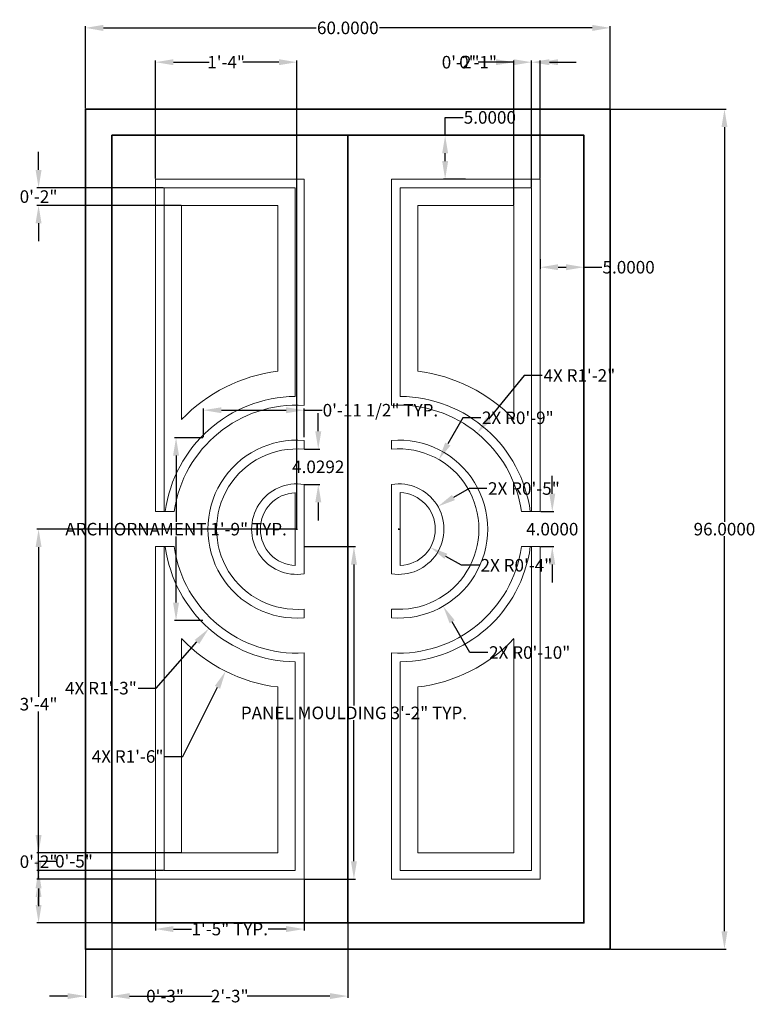
# Model space of a CAD drawing. Units: inches. Extents: x 387 to 471, y 415 to 527.
import ezdxf

# ---------------------------------------------------------------- set-up
doc = ezdxf.new("R2010")
doc.units = ezdxf.units.IN
doc.header["$MEASUREMENT"] = 0
for name, color, linetype, lineweight in [('A-ANNO-DIMS', 2, 'Continuous', 18), ('A-DOOR', 4, 'Continuous', 35), ('A-DOOR-DETL', 3, 'Continuous', 18)]:
    doc.layers.add(name, color=color, linetype=linetype, lineweight=lineweight)
doc.styles.get("Standard").update_dxf_attribs({"font": 'arial.ttf'})
doc.dimstyles.get("Standard").update_dxf_attribs({"dimtxt": 1.433, "dimasz": 2.052, "dimexe": 0.18, "dimexo": 0.0625, "dimgap": 0.09, "dimtad": 0, "dimtih": 1, "dimtoh": 1, "dimdec": 4, "dimzin": 0, "dimdsep": 46, "dimtxsty": 'Standard', "dimcen": 0.09, "dimadec": 0, "dimazin": 0, "dimtfac": 1, "dimtdec": 4, "dimtofl": 0, "dimtmove": 0, "dimatfit": 3, "dimfxl": 1, "dimtolj": 1, "dimtzin": 0, "dimarcsym": 0})

# ---------------------------------------------------------------- blocks, each defined once
blk = doc.blocks.new('*D1')
at = {"layer": 'A-ANNO-DIMS', "color": 0, "lineweight": -2, "transparency": 16777216}
for p, q in [((394.74, 517.13), (394.74, 526.53)), ((396.79, 526.35), (421.12, 526.35)), ((452.69, 526.35), (428.36, 526.35)), ((454.74, 517.13), (454.74, 526.53))]:
    blk.add_line(p, q, dxfattribs=at)
at = {"layer": 'A-ANNO-DIMS', "color": 0, "transparency": 16777216}
for points in [[(396.79, 526.69), (396.79, 526), (394.74, 526.35)], [(452.69, 526.69), (452.69, 526), (454.74, 526.35)]]:
    blk.add_solid(points, dxfattribs=at)
at = {"layer": 'Defpoints', "color": 0, "transparency": 16777216}
for p in [(454.74, 526.35), (394.74, 517.07), (454.74, 517.07)]:
    blk.add_point(p, dxfattribs=at)
at = {"layer": 'A-ANNO-DIMS', "color": 0, "transparency": 16777216, "insert": (424.74, 526.35), "char_height": 1.433, "attachment_point": 5}
blk.add_mtext('\\A1;60.0000', dxfattribs=at)
blk = doc.blocks.new('*D2')
at = {"layer": 'A-ANNO-DIMS', "color": 0, "lineweight": -2, "transparency": 16777216}
for p, q in [((435.87, 514.07), (435.87, 516.12)), ((435.87, 516.12), (437.92, 516.12)), ((438.18, 514.07), (435.69, 514.07)), ((435.87, 511.12), (435.87, 512.02)), ((438.18, 509.07), (435.69, 509.07))]:
    blk.add_line(p, q, dxfattribs=at)
at = {"layer": 'A-ANNO-DIMS', "color": 0, "transparency": 16777216}
for points in [[(435.53, 512.02), (436.21, 512.02), (435.87, 514.07)], [(435.53, 511.12), (436.21, 511.12), (435.87, 509.07)]]:
    blk.add_solid(points, dxfattribs=at)
at = {"layer": 'Defpoints', "color": 0, "transparency": 16777216}
for p in [(435.87, 514.07), (438.24, 514.07), (438.24, 509.07)]:
    blk.add_point(p, dxfattribs=at)
at = {"layer": 'A-ANNO-DIMS', "color": 0, "transparency": 16777216, "insert": (440.98, 516.12), "char_height": 1.433, "attachment_point": 5}
blk.add_mtext('\\A1;5.0000', dxfattribs=at)
blk = doc.blocks.new('*D3')
at = {"layer": 'A-ANNO-DIMS', "color": 0, "lineweight": -2, "transparency": 16777216}
for p, q in [((446.74, 499.93), (446.74, 498.82)), ((451.74, 499.93), (451.74, 498.82)), ((448.79, 499), (449.69, 499)), ((451.74, 499), (453.79, 499))]:
    blk.add_line(p, q, dxfattribs=at)
at = {"layer": 'A-ANNO-DIMS', "color": 0, "transparency": 16777216}
for points in [[(448.79, 499.34), (448.79, 498.66), (446.74, 499)], [(449.69, 499.34), (449.69, 498.66), (451.74, 499)]]:
    blk.add_solid(points, dxfattribs=at)
at = {"layer": 'Defpoints', "color": 0, "transparency": 16777216}
for p in [(446.74, 500), (451.74, 500), (451.74, 499)]:
    blk.add_point(p, dxfattribs=at)
at = {"layer": 'A-ANNO-DIMS', "color": 0, "transparency": 16777216, "insert": (456.85, 499), "char_height": 1.433, "attachment_point": 5}
blk.add_mtext('\\A1;5.0000', dxfattribs=at)
blk = doc.blocks.new('*D4')
at = {"layer": 'A-ANNO-DIMS', "color": 0, "lineweight": -2, "transparency": 16777216}
for p, q in [((448.12, 473.12), (448.12, 475.18)), ((446.8, 471.07), (448.3, 471.07)), ((446.8, 467.07), (448.3, 467.07)), ((448.12, 465.02), (448.12, 462.97))]:
    blk.add_line(p, q, dxfattribs=at)
at = {"layer": 'A-ANNO-DIMS', "color": 0, "transparency": 16777216}
for points in [[(447.78, 473.12), (448.46, 473.12), (448.12, 471.07)], [(447.78, 465.02), (448.46, 465.02), (448.12, 467.07)]]:
    blk.add_solid(points, dxfattribs=at)
at = {"layer": 'Defpoints', "color": 0, "transparency": 16777216}
for p in [(446.74, 471.07), (448.12, 471.07), (446.74, 467.07)]:
    blk.add_point(p, dxfattribs=at)
at = {"layer": 'A-ANNO-DIMS', "color": 0, "transparency": 16777216, "insert": (448.12, 469.07), "char_height": 1.433, "attachment_point": 5}
blk.add_mtext('\\A1;4.0000', dxfattribs=at)
blk = doc.blocks.new('*D5')
at = {"layer": 'A-ANNO-DIMS', "color": 0, "lineweight": -2, "transparency": 16777216}
for p, q in [((454.8, 517.07), (467.99, 517.07)), ((467.81, 515.02), (467.81, 469.89)), ((467.81, 423.12), (467.81, 468.25)), ((454.8, 421.07), (467.99, 421.07))]:
    blk.add_line(p, q, dxfattribs=at)
at = {"layer": 'A-ANNO-DIMS', "color": 0, "transparency": 16777216}
for points in [[(467.47, 515.02), (468.15, 515.02), (467.81, 517.07)], [(467.47, 423.12), (468.15, 423.12), (467.81, 421.07)]]:
    blk.add_solid(points, dxfattribs=at)
at = {"layer": 'Defpoints', "color": 0, "transparency": 16777216}
for p in [(454.74, 517.07), (454.74, 421.07), (467.81, 421.07)]:
    blk.add_point(p, dxfattribs=at)
at = {"layer": 'A-ANNO-DIMS', "color": 0, "transparency": 16777216, "insert": (467.81, 469.07), "char_height": 1.433, "attachment_point": 5}
blk.add_mtext('\\A1;96.0000', dxfattribs=at)
blk = doc.blocks.new('*D6')
at = {"layer": 'A-ANNO-DIMS', "color": 0, "lineweight": -2, "transparency": 16777216}
for p, q in [((421.36, 480.26), (421.36, 482.31)), ((419.8, 478.21), (421.54, 478.21)), ((419.8, 474.18), (421.54, 474.18)), ((421.36, 472.13), (421.36, 470.07))]:
    blk.add_line(p, q, dxfattribs=at)
at = {"layer": 'A-ANNO-DIMS', "color": 0, "transparency": 16777216}
for points in [[(421.02, 480.26), (421.71, 480.26), (421.36, 478.21)], [(421.02, 472.13), (421.71, 472.13), (421.36, 474.18)]]:
    blk.add_solid(points, dxfattribs=at)
at = {"layer": 'Defpoints', "color": 0, "transparency": 16777216}
for p in [(419.74, 478.21), (419.74, 474.18), (421.36, 474.18)]:
    blk.add_point(p, dxfattribs=at)
at = {"layer": 'A-ANNO-DIMS', "color": 0, "transparency": 16777216, "insert": (421.36, 476.19), "char_height": 1.433, "attachment_point": 5}
blk.add_mtext('\\A1;4.0292', dxfattribs=at)
blk = doc.blocks.new('DOOR-PANEL-MOULDING')
for p, q in [((0, 38), (2.14, 38)), ((3, 3), (3, 27.48)), ((16, 24.83), (16, 1)), ((17, 25.85), (17, 0)), ((14, 21.96), (14, 3))]:
    blk.add_line(p, q)
for points in [[(17, 0), (0, 0), (0, 38)], [(16, 1), (1, 1), (1, 38)], [(14, 3), (3, 3)]]:
    blk.add_lwpolyline(points)
for radius, start, end in [(15.17, 187.5743, 269.3464), (14.17, 188.1122, 273.3447), (18.17, 223.5421, 263.1323)]:
    blk.add_arc((16.17, 40), radius, start, end)
blk = doc.blocks.new('DOOR-ARCH-ORNAMENT')
for p, q in [((11, 20.31), (11, 19.31)), ((11, 15.28), (11, 5.07)), ((10, 14.34), (10, 6)), ((11, 1.04), (11, 0.03))]:
    blk.add_line(p, q)
for radius, start, end in [(10.17, 85.3376, 274.6624), (9.17, 84.828, 275.172), (5.17, 80.8019, 279.1981), (4.17, 92.3772, 267.6228)]:
    blk.add_arc((10.17, 10.17), radius, start, end)
blk = doc.blocks.new('*D9')
at = {"layer": 'A-ANNO-DIMS', "color": 0, "lineweight": -2, "transparency": 16777216}
for p, q in [((419.8, 467.07), (425.62, 467.07)), ((425.44, 465.02), (425.44, 448.9)), ((425.44, 431.12), (425.44, 447.24)), ((419.8, 429.07), (425.62, 429.07))]:
    blk.add_line(p, q, dxfattribs=at)
at = {"layer": 'A-ANNO-DIMS', "color": 0, "transparency": 16777216}
for points in [[(425.1, 465.02), (425.78, 465.02), (425.44, 467.07)], [(425.1, 431.12), (425.78, 431.12), (425.44, 429.07)]]:
    blk.add_solid(points, dxfattribs=at)
at = {"layer": 'Defpoints', "color": 0, "transparency": 16777216}
for p in [(419.74, 467.07), (425.44, 467.07), (419.74, 429.07)]:
    blk.add_point(p, dxfattribs=at)
at = {"layer": 'A-ANNO-DIMS', "color": 0, "transparency": 16777216, "insert": (425.44, 448.07), "char_height": 1.433, "attachment_point": 5}
blk.add_mtext('\\A1;PANEL MOULDING 3\'-2" TYP.', dxfattribs=at)
blk = doc.blocks.new('*D10')
at = {"layer": 'A-ANNO-DIMS', "color": 0, "lineweight": -2, "transparency": 16777216}
for p, q in [((402.74, 429.01), (402.74, 423.19)), ((419.74, 429.01), (419.74, 423.19)), ((404.79, 423.37), (406.85, 423.37)), ((417.69, 423.37), (415.63, 423.37))]:
    blk.add_line(p, q, dxfattribs=at)
at = {"layer": 'A-ANNO-DIMS', "color": 0, "transparency": 16777216}
for points in [[(404.79, 423.71), (404.79, 423.03), (402.74, 423.37)], [(417.69, 423.71), (417.69, 423.03), (419.74, 423.37)]]:
    blk.add_solid(points, dxfattribs=at)
at = {"layer": 'Defpoints', "color": 0, "transparency": 16777216}
for p in [(402.74, 429.07), (419.74, 429.07), (419.74, 423.37)]:
    blk.add_point(p, dxfattribs=at)
at = {"layer": 'A-ANNO-DIMS', "color": 0, "transparency": 16777216, "insert": (411.24, 423.37), "char_height": 1.433, "attachment_point": 5}
blk.add_mtext('\\A1;1\'-5" TYP.', dxfattribs=at)
blk = doc.blocks.new('*D11')
at = {"layer": 'A-ANNO-DIMS', "color": 0, "lineweight": -2, "transparency": 16777216}
for p, q in [((408.17, 479.52), (404.92, 479.52)), ((405.1, 477.47), (405.1, 469.9)), ((405.1, 460.67), (405.1, 468.24)), ((408.17, 458.62), (404.92, 458.62))]:
    blk.add_line(p, q, dxfattribs=at)
at = {"layer": 'A-ANNO-DIMS', "color": 0, "transparency": 16777216}
for points in [[(404.76, 477.47), (405.44, 477.47), (405.1, 479.52)], [(404.76, 460.67), (405.44, 460.67), (405.1, 458.62)]]:
    blk.add_solid(points, dxfattribs=at)
at = {"layer": 'Defpoints', "color": 0, "transparency": 16777216}
for p in [(405.1, 479.52), (408.24, 479.52), (408.24, 458.62)]:
    blk.add_point(p, dxfattribs=at)
at = {"layer": 'A-ANNO-DIMS', "color": 0, "transparency": 16777216, "insert": (405.1, 469.07), "char_height": 1.433, "attachment_point": 5}
blk.add_mtext('\\A1;ARCH ORNAMENT 1\'-9" TYP.', dxfattribs=at)
blk = doc.blocks.new('*D12')
at = {"layer": 'A-ANNO-DIMS', "color": 0, "lineweight": -2, "transparency": 16777216}
for p, q in [((408.24, 479.59), (408.24, 482.84)), ((419.74, 479.59), (419.74, 482.84)), ((410.29, 482.66), (417.69, 482.66)), ((419.74, 482.66), (421.79, 482.66))]:
    blk.add_line(p, q, dxfattribs=at)
at = {"layer": 'A-ANNO-DIMS', "color": 0, "transparency": 16777216}
for points in [[(410.29, 483), (410.29, 482.32), (408.24, 482.66)], [(417.69, 483), (417.69, 482.32), (419.74, 482.66)]]:
    blk.add_solid(points, dxfattribs=at)
at = {"layer": 'Defpoints', "color": 0, "transparency": 16777216}
for p in [(419.74, 482.66), (408.24, 479.52), (419.74, 479.52)]:
    blk.add_point(p, dxfattribs=at)
at = {"layer": 'A-ANNO-DIMS', "color": 0, "transparency": 16777216, "insert": (428.47, 482.66), "char_height": 1.433, "attachment_point": 5}
blk.add_mtext('\\A1;0\'-11 1/2" TYP.', dxfattribs=at)
blk = doc.blocks.new('*D13')
at = {"layer": 'A-ANNO-DIMS', "color": 0, "lineweight": -2, "transparency": 16777216}
for p, q in [((397.74, 424.01), (397.74, 415.53)), ((394.74, 421.01), (394.74, 415.53)), ((392.69, 415.71), (390.63, 415.71)), ((399.79, 415.71), (401.84, 415.71))]:
    blk.add_line(p, q, dxfattribs=at)
at = {"layer": 'A-ANNO-DIMS', "color": 0, "transparency": 16777216}
for points in [[(392.69, 416.05), (392.69, 415.37), (394.74, 415.71)], [(399.79, 416.05), (399.79, 415.37), (397.74, 415.71)]]:
    blk.add_solid(points, dxfattribs=at)
at = {"layer": 'Defpoints', "color": 0, "transparency": 16777216}
for p in [(397.74, 424.07), (394.74, 421.07), (397.74, 415.71)]:
    blk.add_point(p, dxfattribs=at)
at = {"layer": 'A-ANNO-DIMS', "color": 0, "transparency": 16777216, "insert": (403.84, 415.71), "char_height": 1.433, "attachment_point": 5}
blk.add_mtext('\\A1;0\'-3"', dxfattribs=at)
blk = doc.blocks.new('*D14')
at = {"layer": 'A-ANNO-DIMS', "color": 0, "lineweight": -2, "transparency": 16777216}
for p, q in [((397.74, 424.01), (397.74, 415.53)), ((424.74, 424.01), (424.74, 415.53)), ((399.79, 415.71), (409.23, 415.71)), ((422.69, 415.71), (413.25, 415.71))]:
    blk.add_line(p, q, dxfattribs=at)
at = {"layer": 'A-ANNO-DIMS', "color": 0, "transparency": 16777216}
for points in [[(399.79, 416.05), (399.79, 415.37), (397.74, 415.71)], [(422.69, 416.05), (422.69, 415.37), (424.74, 415.71)]]:
    blk.add_solid(points, dxfattribs=at)
at = {"layer": 'Defpoints', "color": 0, "transparency": 16777216}
for p in [(397.74, 424.07), (424.74, 424.07), (424.74, 415.71)]:
    blk.add_point(p, dxfattribs=at)
at = {"layer": 'A-ANNO-DIMS', "color": 0, "transparency": 16777216, "insert": (411.24, 415.71), "char_height": 1.433, "attachment_point": 5}
blk.add_mtext('\\A1;2\'-3"', dxfattribs=at)
blk = doc.blocks.new('*D15')
at = {"layer": 'A-ANNO-DIMS', "color": 0, "lineweight": -2, "transparency": 16777216}
for p, q in [((389.38, 429.07), (389.38, 431.12)), ((389.38, 431.12), (391.43, 431.12)), ((402.68, 429.07), (389.2, 429.07)), ((389.38, 426.12), (389.38, 427.02)), ((397.68, 424.07), (389.2, 424.07))]:
    blk.add_line(p, q, dxfattribs=at)
at = {"layer": 'A-ANNO-DIMS', "color": 0, "transparency": 16777216}
for points in [[(389.04, 427.02), (389.72, 427.02), (389.38, 429.07)], [(389.04, 426.12), (389.72, 426.12), (389.38, 424.07)]]:
    blk.add_solid(points, dxfattribs=at)
at = {"layer": 'Defpoints', "color": 0, "transparency": 16777216}
for p in [(389.38, 429.07), (402.74, 429.07), (397.74, 424.07)]:
    blk.add_point(p, dxfattribs=at)
at = {"layer": 'A-ANNO-DIMS', "color": 0, "transparency": 16777216, "insert": (393.43, 431.12), "char_height": 1.433, "attachment_point": 5}
blk.add_mtext('\\A1;0\'-5"', dxfattribs=at)
blk = doc.blocks.new('*D16')
at = {"layer": 'A-ANNO-DIMS', "color": 0, "lineweight": -2, "transparency": 16777216}
for p, q in [((443.69, 522.43), (441.63, 522.43)), ((445.74, 508.13), (445.74, 522.61)), ((446.74, 509.13), (446.74, 522.61)), ((448.79, 522.43), (450.84, 522.43))]:
    blk.add_line(p, q, dxfattribs=at)
at = {"layer": 'A-ANNO-DIMS', "color": 0, "transparency": 16777216}
for points in [[(443.69, 522.77), (443.69, 522.09), (445.74, 522.43)], [(448.79, 522.77), (448.79, 522.09), (446.74, 522.43)]]:
    blk.add_solid(points, dxfattribs=at)
at = {"layer": 'Defpoints', "color": 0, "transparency": 16777216}
for p in [(445.74, 522.43), (446.74, 509.07), (445.74, 508.07)]:
    blk.add_point(p, dxfattribs=at)
at = {"layer": 'A-ANNO-DIMS', "color": 0, "transparency": 16777216, "insert": (439.64, 522.43), "char_height": 1.433, "attachment_point": 5}
blk.add_mtext('\\A1;0\'-1"', dxfattribs=at)
blk = doc.blocks.new('*D17')
at = {"layer": 'A-ANNO-DIMS', "color": 0, "lineweight": -2, "transparency": 16777216}
for p, q in [((441.69, 522.43), (439.63, 522.43)), ((443.74, 506.13), (443.74, 522.61)), ((445.74, 508.13), (445.74, 522.61)), ((447.79, 522.43), (449.84, 522.43))]:
    blk.add_line(p, q, dxfattribs=at)
at = {"layer": 'A-ANNO-DIMS', "color": 0, "transparency": 16777216}
for points in [[(441.69, 522.77), (441.69, 522.09), (443.74, 522.43)], [(447.79, 522.77), (447.79, 522.09), (445.74, 522.43)]]:
    blk.add_solid(points, dxfattribs=at)
at = {"layer": 'Defpoints', "color": 0, "transparency": 16777216}
for p in [(443.74, 522.43), (445.74, 508.07), (443.74, 506.07)]:
    blk.add_point(p, dxfattribs=at)
at = {"layer": 'A-ANNO-DIMS', "color": 0, "transparency": 16777216, "insert": (437.64, 522.43), "char_height": 1.433, "attachment_point": 5}
blk.add_mtext('\\A1;0\'-2"', dxfattribs=at)
blk = doc.blocks.new('*D18')
at = {"layer": 'A-ANNO-DIMS', "color": 0, "lineweight": -2, "transparency": 16777216}
for p, q in [((389.378732, 434.123719), (389.378732, 436.175719)), ((405.676232, 432.071719), (389.198732, 432.071719)), ((403.676232, 430.071719), (389.198732, 430.071719)), ((389.378732, 428.019719), (389.378732, 425.967719))]:
    blk.add_line(p, q, dxfattribs=at)
at = {"layer": 'A-ANNO-DIMS', "color": 0, "transparency": 16777216}
for points in [[(389.036732, 434.123719), (389.720732, 434.123719), (389.378732, 432.071719)], [(389.036732, 428.019719), (389.720732, 428.019719), (389.378732, 430.071719)]]:
    blk.add_solid(points, dxfattribs=at)
at = {"layer": 'Defpoints', "color": 0, "transparency": 16777216}
for p in [(389.378732, 432.071719), (405.738732, 432.071719), (403.738732, 430.071719)]:
    blk.add_point(p, dxfattribs=at)
at = {"layer": 'A-ANNO-DIMS', "color": 0, "transparency": 16777216, "insert": (389.378732, 431.071719), "char_height": 1.433, "attachment_point": 5}
blk.add_mtext('\\A1;0\'-2"', dxfattribs=at)
blk = doc.blocks.new('*D19')
at = {"layer": 'A-ANNO-DIMS', "color": 0, "lineweight": -2, "transparency": 16777216}
for p, q in [((389.378732, 510.123719), (389.378732, 512.175719)), ((403.676232, 508.071719), (389.198732, 508.071719)), ((405.676232, 506.071719), (389.198732, 506.071719)), ((389.378732, 504.019719), (389.378732, 501.967719))]:
    blk.add_line(p, q, dxfattribs=at)
at = {"layer": 'A-ANNO-DIMS', "color": 0, "transparency": 16777216}
for points in [[(389.036732, 510.123719), (389.720732, 510.123719), (389.378732, 508.071719)], [(389.036732, 504.019719), (389.720732, 504.019719), (389.378732, 506.071719)]]:
    blk.add_solid(points, dxfattribs=at)
at = {"layer": 'Defpoints', "color": 0, "transparency": 16777216}
for p in [(403.738732, 508.071719), (389.378732, 506.071719), (405.738732, 506.071719)]:
    blk.add_point(p, dxfattribs=at)
at = {"layer": 'A-ANNO-DIMS', "color": 0, "transparency": 16777216, "insert": (389.378732, 507.071719), "char_height": 1.433, "attachment_point": 5}
blk.add_mtext('\\A1;0\'-2"', dxfattribs=at)
blk = doc.blocks.new('*D20')
at = {"layer": 'A-ANNO-DIMS', "color": 0, "lineweight": -2, "transparency": 16777216}
for p, q in [((402.74, 509.13), (402.74, 522.61)), ((404.79, 522.43), (408.9, 522.43)), ((416.86, 522.43), (412.75, 522.43)), ((418.91, 469.13), (418.91, 522.61))]:
    blk.add_line(p, q, dxfattribs=at)
at = {"layer": 'A-ANNO-DIMS', "color": 0, "transparency": 16777216}
for points in [[(404.79, 522.77), (404.79, 522.09), (402.74, 522.43)], [(416.86, 522.77), (416.86, 522.09), (418.91, 522.43)]]:
    blk.add_solid(points, dxfattribs=at)
at = {"layer": 'Defpoints', "color": 0, "transparency": 16777216}
for p in [(402.74, 522.43), (402.74, 509.07), (418.91, 469.07)]:
    blk.add_point(p, dxfattribs=at)
at = {"layer": 'A-ANNO-DIMS', "color": 0, "transparency": 16777216, "insert": (410.83, 522.43), "char_height": 1.433, "attachment_point": 5}
blk.add_mtext('\\A1;1\'-4"', dxfattribs=at)
blk = doc.blocks.new('*D21')
at = {"layer": 'A-ANNO-DIMS', "color": 0, "lineweight": -2, "transparency": 16777216}
for p, q in [((418.85, 469.07), (389.2, 469.07)), ((389.38, 467.02), (389.38, 449.89)), ((389.38, 431.12), (389.38, 448.25)), ((402.68, 429.07), (389.2, 429.07))]:
    blk.add_line(p, q, dxfattribs=at)
at = {"layer": 'A-ANNO-DIMS', "color": 0, "transparency": 16777216}
for points in [[(389.04, 467.02), (389.72, 467.02), (389.38, 469.07)], [(389.04, 431.12), (389.72, 431.12), (389.38, 429.07)]]:
    blk.add_solid(points, dxfattribs=at)
at = {"layer": 'Defpoints', "color": 0, "transparency": 16777216}
for p in [(418.91, 469.07), (389.38, 429.07), (402.74, 429.07)]:
    blk.add_point(p, dxfattribs=at)
at = {"layer": 'A-ANNO-DIMS', "color": 0, "transparency": 16777216, "insert": (389.38, 449.07), "char_height": 1.433, "attachment_point": 5}
blk.add_mtext('\\A1;3\'-4"', dxfattribs=at)
blk = doc.blocks.new('*D22')
at = {"layer": 'A-ANNO-DIMS', "color": 0, "lineweight": -2, "transparency": 16777216}
for p, q in [((418.82, 469.07), (419, 469.07)), ((418.91, 468.98), (418.91, 469.16)), ((405.86, 443.09), (409.84, 451)), ((403.81, 443.09), (405.86, 443.09))]:
    blk.add_line(p, q, dxfattribs=at)
at = {"layer": 'A-ANNO-DIMS', "color": 0, "transparency": 16777216}
blk.add_solid([(409.53, 451.15), (410.14, 450.84), (410.76, 452.83)], dxfattribs=at)
at = {"layer": 'Defpoints', "color": 0, "transparency": 16777216}
for p in [(418.91, 469.07), (410.76, 452.83)]:
    blk.add_point(p, dxfattribs=at)
at = {"layer": 'A-ANNO-DIMS', "color": 0, "transparency": 16777216, "insert": (399.56, 443.09), "char_height": 1.433, "attachment_point": 5}
blk.add_mtext('\\A1;4X R1\'-6"', dxfattribs=at)
blk = doc.blocks.new('*D23')
at = {"layer": 'A-ANNO-DIMS', "color": 0, "lineweight": -2, "transparency": 16777216}
for p, q in [((418.82, 469.07), (419, 469.07)), ((418.91, 468.98), (418.91, 469.16)), ((402.81, 450.9), (407.49, 456.18)), ((400.76, 450.9), (402.81, 450.9))]:
    blk.add_line(p, q, dxfattribs=at)
at = {"layer": 'A-ANNO-DIMS', "color": 0, "transparency": 16777216}
blk.add_solid([(407.23, 456.41), (407.75, 455.95), (408.85, 457.71)], dxfattribs=at)
at = {"layer": 'Defpoints', "color": 0, "transparency": 16777216}
for p in [(418.91, 469.07), (408.85, 457.71)]:
    blk.add_point(p, dxfattribs=at)
at = {"layer": 'A-ANNO-DIMS', "color": 0, "transparency": 16777216, "insert": (396.51, 450.9), "char_height": 1.433, "attachment_point": 5}
blk.add_mtext('\\A1;4X R1\'-3"', dxfattribs=at)
blk = doc.blocks.new('*D24')
at = {"layer": 'A-ANNO-DIMS', "color": 0, "lineweight": -2, "transparency": 16777216}
for p, q in [((444.92, 486.63), (440.84, 481.63)), ((446.97, 486.63), (444.92, 486.63)), ((430.48, 469.07), (430.66, 469.07)), ((430.57, 468.98), (430.57, 469.16))]:
    blk.add_line(p, q, dxfattribs=at)
at = {"layer": 'A-ANNO-DIMS', "color": 0, "transparency": 16777216}
blk.add_solid([(440.57, 481.85), (441.1, 481.42), (439.54, 480.04)], dxfattribs=at)
at = {"layer": 'Defpoints', "color": 0, "transparency": 16777216}
for p in [(439.54, 480.04), (430.57, 469.07)]:
    blk.add_point(p, dxfattribs=at)
at = {"layer": 'A-ANNO-DIMS', "color": 0, "transparency": 16777216, "insert": (451.22, 486.63), "char_height": 1.433, "attachment_point": 5}
blk.add_mtext('\\A1;4X R1\'-2"', dxfattribs=at)
blk = doc.blocks.new('*D25')
at = {"layer": 'A-ANNO-DIMS', "color": 0, "lineweight": -2, "transparency": 16777216}
for p, q in [((430.48, 469.07), (430.66, 469.07)), ((430.57, 468.98), (430.57, 469.16)), ((438.7, 454.97), (436.68, 458.48)), ((440.75, 454.97), (438.7, 454.97))]:
    blk.add_line(p, q, dxfattribs=at)
at = {"layer": 'A-ANNO-DIMS', "color": 0, "transparency": 16777216}
blk.add_solid([(436.97, 458.65), (436.38, 458.31), (435.65, 460.26)], dxfattribs=at)
at = {"layer": 'Defpoints', "color": 0, "transparency": 16777216}
for p in [(430.57, 469.07), (435.65, 460.26)]:
    blk.add_point(p, dxfattribs=at)
at = {"layer": 'A-ANNO-DIMS', "color": 0, "transparency": 16777216, "insert": (445.54, 454.97), "char_height": 1.433, "attachment_point": 5}
blk.add_mtext('\\A1;2X R0\'-10"', dxfattribs=at)
blk = doc.blocks.new('*D26')
at = {"layer": 'A-ANNO-DIMS', "color": 0, "lineweight": -2, "transparency": 16777216}
for p, q in [((437.9, 481.79), (436.17, 478.8)), ((439.95, 481.79), (437.9, 481.79)), ((430.48, 469.07), (430.66, 469.07)), ((430.57, 468.98), (430.57, 469.16))]:
    blk.add_line(p, q, dxfattribs=at)
at = {"layer": 'A-ANNO-DIMS', "color": 0, "transparency": 16777216}
blk.add_solid([(435.88, 478.97), (436.47, 478.62), (435.15, 477.02)], dxfattribs=at)
at = {"layer": 'Defpoints', "color": 0, "transparency": 16777216}
for p in [(435.15, 477.02), (430.57, 469.07)]:
    blk.add_point(p, dxfattribs=at)
at = {"layer": 'A-ANNO-DIMS', "color": 0, "transparency": 16777216, "insert": (444.18, 481.79), "char_height": 1.433, "attachment_point": 5}
blk.add_mtext('\\A1;2X R0\'-9"', dxfattribs=at)
blk = doc.blocks.new('*D27')
at = {"layer": 'A-ANNO-DIMS', "color": 0, "lineweight": -2, "transparency": 16777216}
for p, q in [((438.6, 473.71), (436.82, 472.68)), ((440.65, 473.71), (438.6, 473.71)), ((430.48, 469.07), (430.66, 469.07)), ((430.57, 468.98), (430.57, 469.16))]:
    blk.add_line(p, q, dxfattribs=at)
at = {"layer": 'A-ANNO-DIMS', "color": 0, "transparency": 16777216}
blk.add_solid([(436.65, 472.98), (436.99, 472.39), (435.05, 471.66)], dxfattribs=at)
at = {"layer": 'Defpoints', "color": 0, "transparency": 16777216}
for p in [(435.05, 471.66), (430.57, 469.07)]:
    blk.add_point(p, dxfattribs=at)
at = {"layer": 'A-ANNO-DIMS', "color": 0, "transparency": 16777216, "insert": (444.88, 473.71), "char_height": 1.433, "attachment_point": 5}
blk.add_mtext('\\A1;2X R0\'-5"', dxfattribs=at)
blk = doc.blocks.new('*D28')
at = {"layer": 'A-ANNO-DIMS', "color": 0, "lineweight": -2, "transparency": 16777216}
for p, q in [((430.48, 469.07), (430.66, 469.07)), ((430.57, 468.98), (430.57, 469.16)), ((437.74, 464.94), (435.96, 465.96)), ((439.79, 464.94), (437.74, 464.94))]:
    blk.add_line(p, q, dxfattribs=at)
at = {"layer": 'A-ANNO-DIMS', "color": 0, "transparency": 16777216}
blk.add_solid([(436.13, 466.26), (435.79, 465.67), (434.18, 466.99)], dxfattribs=at)
at = {"layer": 'Defpoints', "color": 0, "transparency": 16777216}
for p in [(430.57, 469.07), (434.18, 466.99)]:
    blk.add_point(p, dxfattribs=at)
at = {"layer": 'A-ANNO-DIMS', "color": 0, "transparency": 16777216, "insert": (444.02, 464.94), "char_height": 1.433, "attachment_point": 5}
blk.add_mtext('\\A1;2X R0\'-4"', dxfattribs=at)

msp = doc.modelspace()

# ---------------------------------------------------------------- linework, layer by layer
at = {"layer": 'A-DOOR'}
msp.add_line((424.73873, 514.07172), (424.73873, 424.07172), dxfattribs=at)
for points in [[(394.73873, 517.07172), (454.73873, 517.07172), (454.73873, 421.07172), (394.73873, 421.07172)], [(397.73873, 514.07172), (451.73873, 514.07172), (451.73873, 424.07172), (397.73873, 424.07172)]]:
    msp.add_lwpolyline(points, close=True, dxfattribs=at)

# ---------------------------------------------------------------- block references
at = {"layer": 'A-DOOR-DETL', "extrusion": (0, 0, -1), "zscale": -1, "rotation": 180}
msp.add_blockref('DOOR-PANEL-MOULDING', (-402.739, 509.07144), dxfattribs=at)
at = {"layer": 'A-DOOR-DETL', "rotation": 180}
for name, p in [('DOOR-PANEL-MOULDING', (446.73846, 509.07144)), ('DOOR-ARCH-ORNAMENT', (440.73846, 479.24444))]:
    msp.add_blockref(name, p, dxfattribs=at)
at = {"layer": 'A-DOOR-DETL'}
for name, p in [('DOOR-ARCH-ORNAMENT', (408.739, 458.899)), ('DOOR-PANEL-MOULDING', (402.739, 429.072))]:
    msp.add_blockref(name, p, dxfattribs=at)
at = {"layer": 'A-DOOR-DETL', "extrusion": (0, 0, -1), "zscale": -1}
msp.add_blockref('DOOR-PANEL-MOULDING', (-446.73846, 429.072), dxfattribs=at)

# ---------------------------------------------------------------- dimensions: what is measured, and where the dimension line sits
at = {"layer": 'A-ANNO-DIMS'}
for base, p1, p2, override, picture, middle in [((454.73873, 526.34552), (394.73873, 517.07172), (454.73873, 517.07172), {"dimclrd": 0, "dimclre": 0, "dimclrt": 0}, '*D1', (424.73873, 526.34552)), ((402.73873, 522.43172), (418.91182, 469.07172), (402.73873, 509.07172), {"dimdec": 1, "dimlfac": 1, "dimrnd": 0, "dimzin": 1, "dimdsep": 46, "dimlunit": 4, "dimfrac": 2}, '*D20', (410.82528, 522.43172)), ((443.73873, 522.43172), (445.73873, 508.07172), (443.73873, 506.07172), {"dimdec": 1, "dimlfac": 1, "dimrnd": 0, "dimzin": 1, "dimdsep": 46, "dimlunit": 4, "dimfrac": 2}, '*D17', (437.64009, 522.43172)), ((445.73873, 522.43172), (446.73873, 509.07172), (445.73873, 508.07172), {"dimdec": 1, "dimlfac": 1, "dimrnd": 0, "dimzin": 1, "dimdsep": 46, "dimlunit": 4, "dimfrac": 2}, '*D16', (439.64009, 522.43172)), ((451.73873, 499.00173), (446.73873, 499.99566), (451.73873, 499.99566), {"dimclrd": 0, "dimclre": 0, "dimclrt": 0}, '*D3', (456.85279, 499.00173)), ((397.73873, 415.71172), (394.73873, 421.07172), (397.73873, 424.07172), {"dimdec": 1, "dimlfac": 1, "dimrnd": 0, "dimzin": 1, "dimdsep": 46, "dimlunit": 4, "dimfrac": 2}, '*D13', (403.83737, 415.71172)), ((424.73873, 415.71172), (397.73873, 424.07172), (424.73873, 424.07172), {"dimdec": 1, "dimlfac": 1, "dimrnd": 0, "dimzin": 1, "dimdsep": 46, "dimlunit": 4, "dimfrac": 2}, '*D14', (411.23873, 415.71172))]:
    dim = msp.add_linear_dim(base=base, p1=p1, p2=p2, dimstyle='Standard', override=override, dxfattribs=at)
    dim.commit()
    dim.dimension.update_dxf_attribs({"geometry": picture, "text_midpoint": middle})
for base, p1, p2, override, picture, middle in [((435.86883, 514.07172), (438.23873, 509.07172), (438.23873, 514.07172), {"dimclrd": 0, "dimclre": 0, "dimclrt": 0}, '*D2', (440.98289, 516.12372)), ((467.81119, 421.07172), (454.73873, 517.07172), (454.73873, 421.07172), {"dimclrd": 0, "dimclre": 0, "dimclrt": 0}, '*D5', (467.81119, 469.07172)), ((389.37873, 506.07172), (403.73873, 508.07172), (405.73873, 506.07172), {"dimdec": 1, "dimlfac": 1, "dimrnd": 0, "dimzin": 1, "dimdsep": 46, "dimlunit": 4, "dimfrac": 2}, '*D19', (389.37873, 507.07172)), ((421.36448, 474.17829), (419.73873, 478.20746), (419.73873, 474.17829), {"dimclrd": 0, "dimclre": 0, "dimclrt": 0}, '*D6', (421.36448, 476.19288)), ((448.12223, 471.07172), (446.73873, 467.07172), (446.73873, 471.07172), {"dimclrd": 0, "dimclre": 0, "dimclrt": 0}, '*D4', (448.12223, 469.07172)), ((389.37873, 429.07172), (418.91182, 469.07172), (402.73873, 429.07172), {"dimdec": 1, "dimlfac": 1, "dimrnd": 0, "dimzin": 1, "dimdsep": 46, "dimlunit": 4, "dimfrac": 2}, '*D21', (389.37873, 449.07172)), ((389.37873, 432.07172), (403.73873, 430.07172), (405.73873, 432.07172), {"dimdec": 1, "dimlfac": 1, "dimrnd": 0, "dimzin": 1, "dimdsep": 46, "dimlunit": 4, "dimfrac": 2}, '*D18', (389.37873, 431.07172)), ((389.37873, 429.07172), (397.73873, 424.07172), (402.73873, 429.07172), {"dimdec": 1, "dimlfac": 1, "dimrnd": 0, "dimzin": 1, "dimdsep": 46, "dimlunit": 4, "dimfrac": 2}, '*D15', (393.42537, 431.12372))]:
    dim = msp.add_linear_dim(base=base, p1=p1, p2=p2, angle=90, dimstyle='Standard', override=override, dxfattribs=at)
    dim.commit()
    dim.dimension.update_dxf_attribs({"geometry": picture, "text_midpoint": middle})
for center, mpoint, text, picture, middle in [((430.56564, 469.07172), (439.53701, 480.04401), '4X <>', '*D24', (451.22056, 486.62738)), ((430.56564, 469.07172), (435.14875, 477.01783), '2X <>', '*D26', (444.18273, 481.7855)), ((418.91182, 469.07172), (408.84984, 457.71482), '4X <>', '*D23', (396.51192, 450.90068)), ((418.91182, 469.07172), (410.75701, 452.83102), '4X <>', '*D22', (399.56339, 443.0866)), ((430.56564, 469.07172), (435.64987, 460.26023), '2X <>', '*D25', (445.5412, 454.97333))]:
    dim = msp.add_radius_dim(center=center, mpoint=mpoint, text=text, dimstyle='Standard', override={"dimdec": 1, "dimlfac": 1, "dimrnd": 0, "dimzin": 1, "dimdsep": 46, "dimlunit": 4, "dimfrac": 2}, dxfattribs=at)
    dim.commit()
    dim.dimension.update_dxf_attribs({"geometry": picture, "text_midpoint": middle, "dimtype": 164})
for base, p1, p2, picture, middle in [((419.73873, 482.65794), (408.23736, 479.52266), (419.73873, 479.52266), '*D12', (428.47439, 482.65794)), ((419.73873, 423.37172), (402.73873, 429.07172), (419.73873, 429.07172), '*D10', (411.23873, 423.37172))]:
    dim = msp.add_linear_dim(base=base, p1=p1, p2=p2, text='<> TYP.', dimstyle='Standard', override={"dimdec": 1, "dimrnd": 0, "dimzin": 1, "dimlunit": 4, "dimfrac": 2}, dxfattribs=at)
    dim.commit()
    dim.dimension.update_dxf_attribs({"geometry": picture, "text_midpoint": middle})
for base, p1, p2, text, picture, middle in [((405.10207, 479.52266), (408.23736, 458.62078), (408.23736, 479.52266), 'ARCH ORNAMENT <> TYP.', '*D11', (405.10207, 469.07172)), ((425.43873, 467.07172), (419.73873, 429.07172), (419.73873, 467.07172), 'PANEL MOULDING <> TYP.', '*D9', (425.43873, 448.07172))]:
    dim = msp.add_linear_dim(base=base, p1=p1, p2=p2, angle=90, text=text, dimstyle='Standard', override={"dimdec": 1, "dimrnd": 0, "dimzin": 1, "dimlunit": 4, "dimfrac": 2}, dxfattribs=at)
    dim.commit()
    dim.dimension.update_dxf_attribs({"geometry": picture, "text_midpoint": middle})
for mpoint, picture, middle in [((435.046, 471.65769), '*D27', (444.88454, 473.70924)), ((434.18182, 466.98895), '*D28', (444.02225, 464.94067))]:
    dim = msp.add_radius_dim(center=(430.56564, 469.07172), mpoint=mpoint, text='2X <>', dimstyle='Standard', override={"dimdec": 1, "dimlfac": 1, "dimrnd": 0, "dimzin": 1, "dimdsep": 46, "dimlunit": 4, "dimfrac": 2}, dxfattribs=at)
    dim.commit()
    dim.dimension.update_dxf_attribs({"geometry": picture, "text_midpoint": middle})

doc.saveas('drawing.dxf')
